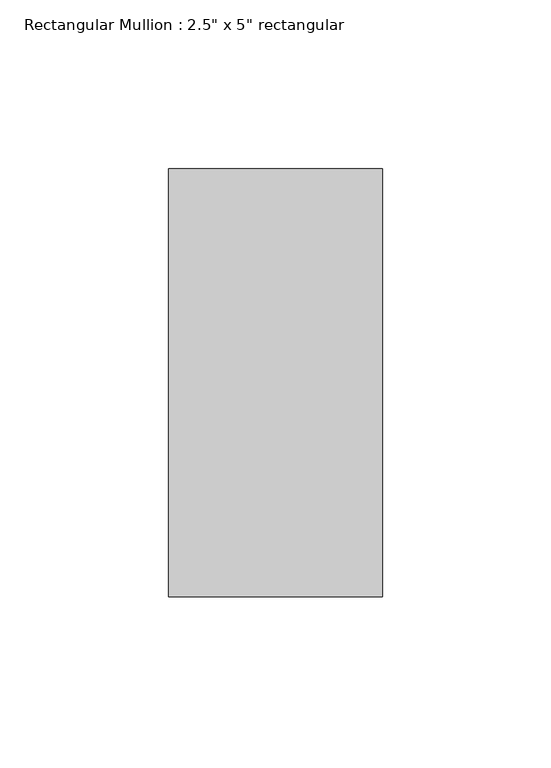
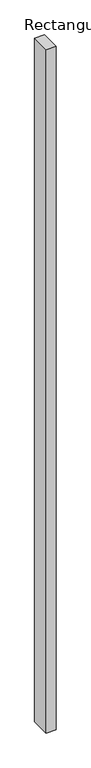
"""IFC4 building model written with IfcOpenShell, lengths in millimetres: member geometry."""

from ifc_helpers import new_model, si_unit, frame, origin, place, context, project, spatial, polyline, outline, extrude, source, transform, mapped, element, save


def member_4d280e20(model_context):
    return source(origin(), model_context, "Body", "SweptSolid", [
        extrude(outline(polyline([(0.0, 63.5), (0.0, -63.5), (-63.5, -63.5), (-63.5, 63.5), (0.0, 63.5)])), frame((0.0, 0.0, -4635.5), z_axis=(0.0, 0.0, 1.0), x_axis=(1.0, 0.0, 0.0)), (0.0, 0.0, 1.0), 4635.5),
    ])


if __name__ == "__main__":
    model = new_model("IFC4")
    model_context = context("Model", 3, world=origin())
    ifc_project = project(units=[si_unit("LENGTHUNIT", "METRE", prefix="MILLI")], contexts=[model_context])
    site = spatial("IfcSite", under=ifc_project)
    building = spatial("IfcBuilding", under=site)
    placement = place(None, origin())
    member_shape = member_4d280e20(model_context)
    element("IfcMember", 1, ObjectType="Rectangular Mullion : 2.5\" x 5\" rectangular", at=placement, inside=building, context=model_context, shape_type="MappedRepresentation", body=[
        mapped(member_shape, transform((0.0, 0.0, 0.0), x_axis=(1.0, 0.0, 0.0), y_axis=(0.0, 1.0, 0.0), z_axis=(0.0, 0.0, 1.0))),
    ])
    save(model, "model.ifc")

# Revit data of these elements
# Type "Rectangular Mullion : 2.5\" x 5\" rectangular"
#   built-in parameter 1007304 = 0.416667 (stored number, unit not read)
#   built-in parameter 1007301 = 0.104167 (stored number, unit not read)
#   built-in parameter 1007300 = 0.104167 (stored number, unit not read)
# Element 1 (IfcMember, "Rectangular Mullion : 2.5\" x 5\" rectangular")
#   Materials on its faces: "Aluminum"
# Materials
#   "Aluminum": class "Metal", colour RGB 247 247 247, transparency 0, Description = "Aluminum 6061", Cost = 0
